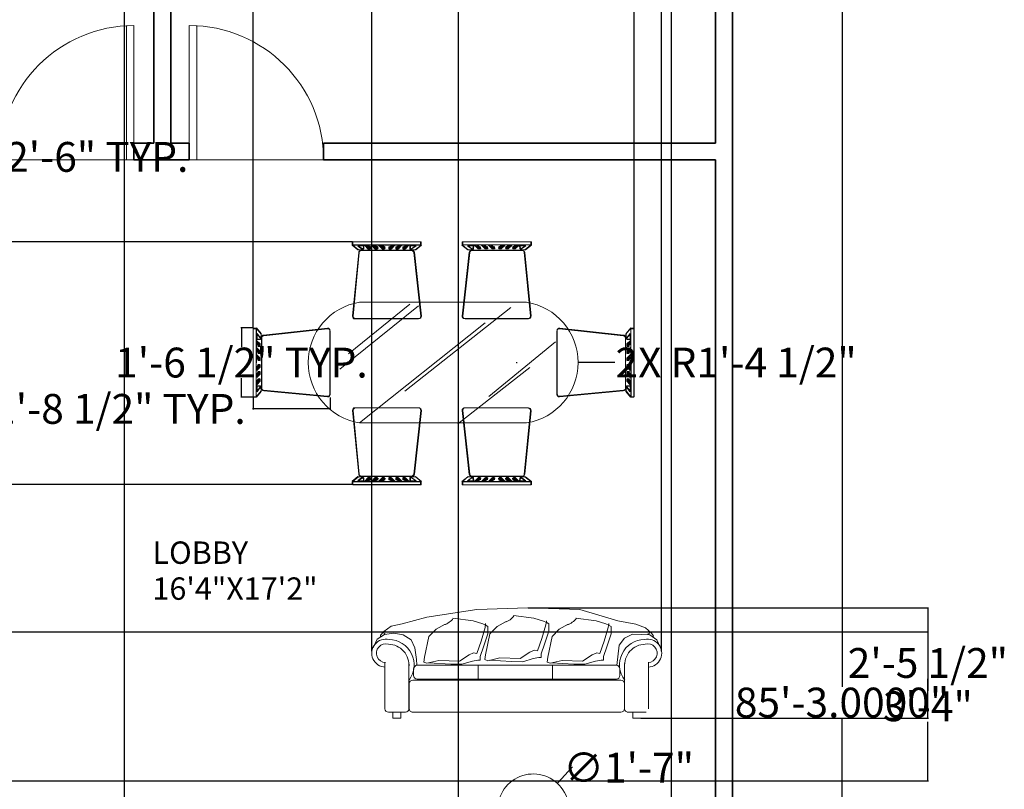
# Model space of a CAD drawing. Units: inches. Extents: x -438 to 102, y -60 to 1091.
# Tile 5 of 20: x -162 to 102, y 492 to 699. Entities that reach past the tile are written whole.
import ezdxf

# ---------------------------------------------------------------- set-up
doc = ezdxf.new("R2010")
doc.units = ezdxf.units.IN
doc.header["$MEASUREMENT"] = 0
for name, color, linetype, lineweight, true_color in [('A-ANNO-DIMS', 217, 'Continuous', 18, 0x93278f), ('A-DOOR', 30, 'Continuous', 18, 0xf26722), ('A-WALL', 2, 'Continuous', 35, 0xf1eb1f), ('C-PROP', 2, 'Continuous', 35, 0xf1eb1f)]:
    doc.layers.add(name, color=color, linetype=linetype, lineweight=lineweight, true_color=true_color)
doc.layers.add('A-AREA-IDEN', color=4, linetype='Continuous', lineweight=18)
doc.layers.add('Furniture', color=7, linetype='Continuous', lineweight=15)
doc.styles.get("Standard").update_dxf_attribs({"font": 'arial.ttf'})
doc.dimstyles.get("Standard").update_dxf_attribs({"dimtxt": 8, "dimasz": 0.18, "dimexe": 0.18, "dimexo": 0.0625, "dimgap": 0.09, "dimtad": 0, "dimtih": 1, "dimtoh": 1, "dimdec": 4, "dimzin": 0, "dimdsep": 46, "dimlunit": 3, "dimtxsty": 'Standard', "dimcen": 0.09, "dimadec": 0, "dimazin": 0, "dimtfac": 1, "dimtdec": 4, "dimtofl": 0, "dimtmove": 0, "dimatfit": 3, "dimfxl": 1, "dimtolj": 1, "dimtzin": 0, "dimarcsym": 0})

# ---------------------------------------------------------------- blocks, each defined once
blk = doc.blocks.new('*D5')
at = {"layer": 'A-ANNO-DIMS', "color": 0, "lineweight": -2, "transparency": 16777216}
for p, q in [((28.92, 1027), (58.42, 1027)), ((58.24, 1026.82), (58.24, 519.68)), ((58.24, 4.18), (58.24, 511.32)), ((28.92, 4), (58.42, 4))]:
    blk.add_line(p, q, dxfattribs=at)
at = {"layer": 'A-ANNO-DIMS', "color": 0, "transparency": 16777216}
for points in [[(58.21, 1026.82), (58.27, 1026.82), (58.24, 1027)], [(58.21, 4.18), (58.27, 4.18), (58.24, 4)]]:
    blk.add_solid(points, dxfattribs=at)
at = {"layer": 'Defpoints', "color": 0, "transparency": 16777216}
for p in [(28.85, 1027), (28.85, 4), (58.24, 4)]:
    blk.add_point(p, dxfattribs=at)
at = {"layer": 'A-ANNO-DIMS', "color": 0, "transparency": 16777216, "insert": (58.24, 515.5), "char_height": 8, "attachment_point": 5}
blk.add_mtext('\\A1;85\'-3.0000"', dxfattribs=at)
blk = doc.blocks.new('DOOR-SWING-36')
for p, q in [((-36, 0), (0, 0)), ((-2, 0), (-2, -36)), ((0, 0), (0, -36))]:
    blk.add_line(p, q)
blk.add_arc((0, 0), 36, 180, 270)
blk = doc.blocks.new('CHAIR-DINING')
for p, q in [((-10.32, -8.58, -3.57), (-10.34, 8.44, -3.57)), ((-10.26, -8.42, -3.57), (-10.28, 8.6, -3.57)), ((-9.64, 9.07, -3.57), (7.45, 7.21, -3.57)), ((-9.58, 9.23, -3.57), (7.51, 7.37, -3.57)), ((9.39, 9.16, -3.57), (8.13, 7.59, -3.57)), ((9.45, 9.32, -3.57), (8.19, 7.75, -3.57)), ((10.27, 9.04, -3.57), (9.45, 9.03, -3.57)), ((9.45, 9.03, -3.57), (9.47, -9.32, -3.57)), ((10.33, 9.2, -3.57), (9.51, 9.2, -3.57)), ((9.51, 9.2, -3.57), (9.53, -9.16, -3.57)), ((10.28, -9.32, -3.57), (10.27, 9.04, -3.57)), ((10.34, -9.16, -3.57), (10.33, 9.2, -3.57)), ((8.01, 6.58, -3.57), (8.02, -6.93, -3.57)), ((8.07, 6.75, -3.57), (8.08, -6.76, -3.57)), ((8.13, 7.59, -3.57), (8.2, 6.27, -3.57)), ((8.19, 7.75, -3.57), (8.25, 6.43, -3.57)), ((8.2, 6.27, -3.57), (9.2, 7.65, -3.57)), ((8.25, 6.43, -3.57), (9.26, 7.81, -3.57)), ((9.26, 6.14, -3.57), (8.38, 6.2, -3.57)), ((9.33, 5.77, -3.57), (8.39, 4.82, -3.57)), ((9.32, 6.3, -3.57), (8.44, 6.37, -3.57)), ((9.39, 5.93, -3.57), (8.44, 4.98, -3.57)), ((8.45, 4.48, -3.57), (9.32, 5.43, -3.57)), ((9.2, 7.65, -3.57), (9.26, 6.14, -3.57)), ((9.26, 7.81, -3.57), (9.32, 6.3, -3.57)), ((9.32, 5.43, -3.57), (9.32, 5.05, -3.57)), ((8.39, 4.32, -3.57), (9.26, 5.26, -3.57)), ((8.39, 4.82, -3.57), (8.39, 4.32, -3.57)), ((9.33, 3.88, -3.57), (8.39, 2.94, -3.57)), ((8.39, 2.43, -3.57), (9.27, 3.38, -3.57)), ((8.39, 2.94, -3.57), (8.39, 2.43, -3.57)), ((8.44, 4.98, -3.57), (8.45, 4.48, -3.57)), ((9.01, 4.32, -3.57), (8.45, 4.26, -3.57)), ((9.39, 4.04, -3.57), (8.45, 3.1, -3.57)), ((8.45, 2.6, -3.57), (9.33, 3.54, -3.57)), ((8.45, 3.1, -3.57), (8.45, 2.6, -3.57)), ((9.07, 4.48, -3.57), (8.51, 4.42, -3.57)), ((9.26, 4.89, -3.57), (8.89, 4.45, -3.57)), ((8.89, 4.45, -3.57), (9.01, 4.32, -3.57)), ((9.27, 3, -3.57), (8.89, 2.56, -3.57)), ((9.32, 5.05, -3.57), (8.95, 4.61, -3.57)), ((8.95, 4.61, -3.57), (9.07, 4.48, -3.57)), ((9.33, 3.16, -3.57), (8.95, 2.72, -3.57)), ((8.95, 2.72, -3.57), (9.08, 2.6, -3.57)), ((9.26, 5.26, -3.57), (9.26, 4.89, -3.57)), ((9.27, 3.38, -3.57), (9.27, 3, -3.57)), ((9.33, 3.54, -3.57), (9.33, 3.16, -3.57)), ((9.33, 1.99, -3.57), (8.39, 1.05, -3.57)), ((8.39, 0.55, -3.57), (9.27, 1.49, -3.57)), ((8.39, 1.05, -3.57), (8.39, 0.55, -3.57)), ((9.02, 2.43, -3.57), (8.45, 2.37, -3.57)), ((9.39, 2.16, -3.57), (8.45, 1.21, -3.57)), ((8.45, 0.71, -3.57), (9.33, 1.65, -3.57)), ((8.45, 1.21, -3.57), (8.45, 0.71, -3.57)), ((9.02, 0.55, -3.57), (8.45, 0.49, -3.57)), ((9.08, 2.6, -3.57), (8.51, 2.53, -3.57)), ((9.08, 0.71, -3.57), (8.51, 0.65, -3.57)), ((8.89, 2.56, -3.57), (9.02, 2.43, -3.57)), ((9.27, 1.11, -3.57), (8.89, 0.67, -3.57)), ((8.89, 0.67, -3.57), (9.02, 0.55, -3.57)), ((9.33, 1.28, -3.57), (8.95, 0.84, -3.57)), ((8.95, 0.84, -3.57), (9.08, 0.71, -3.57)), ((9.27, 1.49, -3.57), (9.27, 1.11, -3.57)), ((9.33, 1.65, -3.57), (9.33, 1.28, -3.57)), ((8.39, -1.21, -3.57), (8.39, -0.71, -3.57)), ((8.39, -0.71, -3.57), (9.27, -1.65, -3.57)), ((9.33, -2.15, -3.57), (8.39, -1.21, -3.57)), ((8.39, -3.1, -3.57), (8.39, -2.59, -3.57)), ((8.39, -2.59, -3.57), (9.27, -3.54, -3.57)), ((8.45, -1.05, -3.57), (8.45, -0.55, -3.57)), ((8.45, -0.55, -3.57), (9.33, -1.49, -3.57)), ((9.02, -0.71, -3.57), (8.45, -0.65, -3.57)), ((9.39, -1.99, -3.57), (8.45, -1.05, -3.57)), ((8.45, -2.94, -3.57), (8.45, -2.43, -3.57)), ((8.45, -2.43, -3.57), (9.33, -3.37, -3.57)), ((9.02, -2.59, -3.57), (8.45, -2.53, -3.57)), ((9.08, -0.55, -3.57), (8.51, -0.48, -3.57)), ((9.08, -2.43, -3.57), (8.51, -2.37, -3.57)), ((8.89, -0.83, -3.57), (9.02, -0.71, -3.57)), ((9.27, -1.27, -3.57), (8.89, -0.83, -3.57)), ((8.89, -2.72, -3.57), (9.02, -2.59, -3.57)), ((8.95, -0.67, -3.57), (9.08, -0.55, -3.57)), ((9.33, -1.11, -3.57), (8.95, -0.67, -3.57)), ((8.95, -2.56, -3.57), (9.08, -2.43, -3.57)), ((9.33, -3, -3.57), (8.95, -2.56, -3.57)), ((9.27, -1.65, -3.57), (9.27, -1.27, -3.57)), ((9.33, -1.49, -3.57), (9.33, -1.11, -3.57)), ((9.34, -4.04, -3.57), (8.39, -3.1, -3.57)), ((8.39, -4.98, -3.57), (8.39, -4.48, -3.57)), ((8.39, -4.48, -3.57), (9.27, -5.42, -3.57)), ((9.34, -5.93, -3.57), (8.39, -4.98, -3.57)), ((9.39, -3.88, -3.57), (8.45, -2.94, -3.57)), ((8.45, -4.82, -3.57), (8.45, -4.32, -3.57)), ((8.45, -4.32, -3.57), (9.33, -5.26, -3.57)), ((9.4, -5.76, -3.57), (8.45, -4.82, -3.57)), ((9.02, -4.48, -3.57), (8.46, -4.42, -3.57)), ((9.08, -4.32, -3.57), (8.52, -4.26, -3.57)), ((9.27, -3.16, -3.57), (8.89, -2.72, -3.57)), ((8.9, -4.61, -3.57), (9.02, -4.48, -3.57)), ((9.27, -5.05, -3.57), (8.9, -4.61, -3.57)), ((8.96, -4.44, -3.57), (9.08, -4.32, -3.57)), ((9.33, -4.88, -3.57), (8.96, -4.44, -3.57)), ((9.27, -3.54, -3.57), (9.27, -3.16, -3.57)), ((9.27, -5.42, -3.57), (9.27, -5.05, -3.57)), ((9.33, -3.37, -3.57), (9.33, -3, -3.57)), ((9.33, -5.26, -3.57), (9.33, -4.88, -3.57)), ((7.45, -7.55, -3.57), (-9.64, -9.21, -3.57)), ((7.51, -7.39, -3.57), (-9.58, -9.04, -3.57)), ((8.14, -7.75, -3.57), (8.21, -6.43, -3.57)), ((9.4, -9.32, -3.57), (8.14, -7.75, -3.57)), ((8.2, -7.59, -3.57), (8.27, -6.27, -3.57)), ((9.46, -9.16, -3.57), (8.2, -7.59, -3.57)), ((8.21, -6.43, -3.57), (9.21, -7.81, -3.57)), ((8.27, -6.27, -3.57), (9.27, -7.65, -3.57)), ((9.27, -6.3, -3.57), (8.39, -6.37, -3.57)), ((9.33, -6.14, -3.57), (8.45, -6.2, -3.57)), ((9.21, -7.81, -3.57), (9.27, -6.3, -3.57)), ((9.27, -7.65, -3.57), (9.33, -6.14, -3.57)), ((9.47, -9.32, -3.57), (10.28, -9.32, -3.57)), ((9.53, -9.16, -3.57), (10.34, -9.16, -3.57))]:
    blk.add_line(p, q)
for centre, start, end in [((-9.71, 8.44, -3.57), 83.7931, 180.0502), ((-9.65, 8.6, -3.57), 83.7931, 180.0502), ((7.38, 6.58, -3.57), 0.0502, 83.7931), ((7.44, 6.75, -3.57), 0.0502, 83.7931), ((7.39, -6.93, -3.57), 275.5303, 0.0502), ((7.45, -6.76, -3.57), 275.5303, 0.0502), ((-9.7, -8.58, -3.57), 180.0502, 275.5303), ((-9.64, -8.42, -3.57), 180.0502, 275.5303)]:
    blk.add_arc(centre, 0.629, start, end)
blk = doc.blocks.new('*D14')
at = {"layer": 'A-ANNO-DIMS', "color": 0, "lineweight": -2, "transparency": 16777216}
for p, q in [((-99.6, 597.28), (-99.6, 594.06)), ((-78.92, 597.28), (-78.92, 594.06)), ((-99.6, 594.24), (-99.78, 594.24)), ((-79.1, 594.24), (-99.42, 594.24))]:
    blk.add_line(p, q, dxfattribs=at)
at = {"layer": 'A-ANNO-DIMS', "color": 0, "transparency": 16777216}
for points in [[(-99.42, 594.27), (-99.42, 594.21), (-99.6, 594.24)], [(-79.1, 594.27), (-79.1, 594.21), (-78.92, 594.24)]]:
    blk.add_solid(points, dxfattribs=at)
at = {"layer": 'Defpoints', "color": 0, "transparency": 16777216}
for p in [(-99.6, 597.34), (-78.92, 597.34), (-99.6, 594.24)]:
    blk.add_point(p, dxfattribs=at)
at = {"layer": 'A-ANNO-DIMS', "color": 0, "transparency": 16777216, "insert": (-152.46, 594.24), "char_height": 8, "attachment_point": 5}
blk.add_mtext('\\A1;CHAIR 1\'-8 1/2" TYP.', dxfattribs=at)
blk = doc.blocks.new('*D15')
at = {"layer": 'A-ANNO-DIMS', "color": 0, "lineweight": -2, "transparency": 16777216}
for p, q in [((-99.66, 615.98), (-102.88, 615.98)), ((-102.7, 615.8), (-102.7, 610.89)), ((-102.7, 597.52), (-102.7, 602.44)), ((-99.66, 597.34), (-102.88, 597.34))]:
    blk.add_line(p, q, dxfattribs=at)
at = {"layer": 'A-ANNO-DIMS', "color": 0, "transparency": 16777216}
for points in [[(-102.73, 615.8), (-102.67, 615.8), (-102.7, 615.98)], [(-102.73, 597.52), (-102.67, 597.52), (-102.7, 597.34)]]:
    blk.add_solid(points, dxfattribs=at)
at = {"layer": 'Defpoints', "color": 0, "transparency": 16777216}
for p in [(-102.7, 615.98), (-99.6, 615.98), (-99.6, 597.34)]:
    blk.add_point(p, dxfattribs=at)
at = {"layer": 'A-ANNO-DIMS', "color": 0, "transparency": 16777216, "insert": (-102.7, 606.66), "char_height": 8, "attachment_point": 5}
blk.add_mtext('\\A1;1\'-6 1/2" TYP.', dxfattribs=at)
blk = doc.blocks.new('*D22')
at = {"layer": 'A-ANNO-DIMS', "color": 0, "lineweight": -2, "transparency": 16777216}
for p, q in [((-230.65, 657.36), (-230.65, 661.98)), ((-230.47, 661.8), (-200.83, 661.8)), ((-200.65, 657.36), (-200.65, 661.98)), ((-200.65, 661.8), (-200.47, 661.8))]:
    blk.add_line(p, q, dxfattribs=at)
at = {"layer": 'A-ANNO-DIMS', "color": 0, "transparency": 16777216}
for points in [[(-230.47, 661.83), (-230.47, 661.77), (-230.65, 661.8)], [(-200.83, 661.83), (-200.83, 661.77), (-200.65, 661.8)]]:
    blk.add_solid(points, dxfattribs=at)
at = {"layer": 'Defpoints', "color": 0, "transparency": 16777216}
for p in [(-200.65, 661.8), (-230.65, 657.3), (-200.65, 657.3)]:
    blk.add_point(p, dxfattribs=at)
at = {"layer": 'A-ANNO-DIMS', "color": 0, "transparency": 16777216, "insert": (-157.88, 661.8), "char_height": 8, "attachment_point": 5}
blk.add_mtext('\\A1;DOOR 2\'-6" TYP.', dxfattribs=at)
blk = doc.blocks.new('*D37')
at = {"layer": 'A-ANNO-DIMS', "color": 0, "lineweight": -2, "transparency": 16777216}
for p, q in [((-179.8, 234.94), (-179.8, 1079.58)), ((-179.62, 1079.4), (-176.98, 1079.4)), ((-134.26, 1079.4), (-136.9, 1079.4)), ((-134.08, 234.94), (-134.08, 1079.58))]:
    blk.add_line(p, q, dxfattribs=at)
at = {"layer": 'A-ANNO-DIMS', "color": 0, "transparency": 16777216}
for points in [[(-179.62, 1079.43), (-179.62, 1079.37), (-179.8, 1079.4)], [(-134.26, 1079.43), (-134.26, 1079.37), (-134.08, 1079.4)]]:
    blk.add_solid(points, dxfattribs=at)
at = {"layer": 'Defpoints', "color": 0, "transparency": 16777216}
for p in [(-134.08, 1079.4), (-179.8, 234.88), (-134.08, 234.88)]:
    blk.add_point(p, dxfattribs=at)
at = {"layer": 'A-ANNO-DIMS', "color": 0, "transparency": 16777216, "insert": (-156.94, 1079.4), "char_height": 8, "attachment_point": 5}
blk.add_mtext('\\A1;3\'-9 1/2"', dxfattribs=at)
blk = doc.blocks.new('*D45')
at = {"layer": 'A-ANNO-DIMS', "color": 0, "lineweight": -2, "transparency": 16777216}
for p, q in [((-99.58, 615.92), (-99.58, 1079.58)), ((-99.4, 1079.4), (-59.27, 1079.4)), ((2.32, 1079.4), (-37.82, 1079.4)), ((2.5, 615.92), (2.5, 1079.58))]:
    blk.add_line(p, q, dxfattribs=at)
at = {"layer": 'A-ANNO-DIMS', "color": 0, "transparency": 16777216}
for points in [[(-99.4, 1079.43), (-99.4, 1079.37), (-99.58, 1079.4)], [(2.32, 1079.43), (2.32, 1079.37), (2.5, 1079.4)]]:
    blk.add_solid(points, dxfattribs=at)
at = {"layer": 'Defpoints', "color": 0, "transparency": 16777216}
for p in [(2.5, 1079.4), (-99.58, 615.86), (2.5, 615.86)]:
    blk.add_point(p, dxfattribs=at)
at = {"layer": 'A-ANNO-DIMS', "color": 0, "transparency": 16777216, "insert": (-48.54, 1079.4), "char_height": 8, "attachment_point": 5}
blk.add_mtext('\\A1;8\'-6"', dxfattribs=at)
blk = doc.blocks.new('*D46')
at = {"layer": 'A-ANNO-DIMS', "color": 0, "lineweight": -2, "transparency": 16777216}
for p, q in [((-72.95, 639.04), (-414.94, 639.04)), ((-414.76, 638.86), (-414.76, 610.65)), ((-414.76, 574.12), (-414.76, 602.33)), ((-73.11, 573.94), (-414.94, 573.94))]:
    blk.add_line(p, q, dxfattribs=at)
at = {"layer": 'A-ANNO-DIMS', "color": 0, "transparency": 16777216}
for points in [[(-414.79, 638.86), (-414.73, 638.86), (-414.76, 639.04)], [(-414.79, 574.12), (-414.73, 574.12), (-414.76, 573.94)]]:
    blk.add_solid(points, dxfattribs=at)
at = {"layer": 'Defpoints', "color": 0, "transparency": 16777216}
for p in [(-414.76, 639.04), (-72.89, 639.04), (-73.05, 573.94)]:
    blk.add_point(p, dxfattribs=at)
at = {"layer": 'A-ANNO-DIMS', "color": 0, "transparency": 16777216, "insert": (-414.76, 606.49), "char_height": 8, "attachment_point": 5}
blk.add_mtext('\\A1;5\'-5"', dxfattribs=at)
blk = doc.blocks.new('*D47')
at = {"layer": 'A-ANNO-DIMS', "color": 0, "lineweight": -2, "transparency": 16777216}
for p, q in [((-67.74, 529.33), (-67.74, 1079.58)), ((-67.56, 1079.4), (-48.98, 1079.4)), ((9.73, 1079.4), (-8.85, 1079.4)), ((9.91, 529.33), (9.91, 1079.58))]:
    blk.add_line(p, q, dxfattribs=at)
at = {"layer": 'A-ANNO-DIMS', "color": 0, "transparency": 16777216}
for points in [[(-67.56, 1079.43), (-67.56, 1079.37), (-67.74, 1079.4)], [(9.73, 1079.43), (9.73, 1079.37), (9.91, 1079.4)]]:
    blk.add_solid(points, dxfattribs=at)
at = {"layer": 'Defpoints', "color": 0, "transparency": 16777216}
for p in [(9.91, 1079.4), (-67.74, 529.27), (9.91, 529.27)]:
    blk.add_point(p, dxfattribs=at)
at = {"layer": 'A-ANNO-DIMS', "color": 0, "transparency": 16777216, "insert": (-28.91, 1079.4), "char_height": 8, "attachment_point": 5}
blk.add_mtext('\\A1;6\'-5 1/2"', dxfattribs=at)
blk = doc.blocks.new('*D48')
at = {"layer": 'A-ANNO-DIMS', "color": 0, "lineweight": -2, "transparency": 16777216}
for p, q in [((-25.85, 540.93), (81.43, 540.93)), ((81.25, 540.75), (81.25, 530.34)), ((81.25, 511.48), (81.25, 521.89)), ((4.34, 511.3), (81.43, 511.3))]:
    blk.add_line(p, q, dxfattribs=at)
at = {"layer": 'A-ANNO-DIMS', "color": 0, "transparency": 16777216}
for points in [[(81.22, 540.75), (81.28, 540.75), (81.25, 540.93)], [(81.22, 511.48), (81.28, 511.48), (81.25, 511.3)]]:
    blk.add_solid(points, dxfattribs=at)
at = {"layer": 'Defpoints', "color": 0, "transparency": 16777216}
for p in [(-25.91, 540.93), (4.28, 511.3), (81.25, 511.3)]:
    blk.add_point(p, dxfattribs=at)
at = {"layer": 'A-ANNO-DIMS', "color": 0, "transparency": 16777216, "insert": (81.25, 526.12), "char_height": 8, "attachment_point": 5}
blk.add_mtext('\\A1;2\'-5 1/2"', dxfattribs=at)
blk = doc.blocks.new('*D49')
at = {"layer": 'A-ANNO-DIMS', "color": 0, "lineweight": -2, "transparency": 16777216}
for p, q in [((-44.57, 339.86), (-44.57, 1079.58)), ((-44.39, 1079.4), (-26.89, 1079.4)), ((12.37, 1079.4), (-5.13, 1079.4)), ((12.55, 312.51), (12.55, 1079.58))]:
    blk.add_line(p, q, dxfattribs=at)
at = {"layer": 'A-ANNO-DIMS', "color": 0, "transparency": 16777216}
for points in [[(-44.39, 1079.43), (-44.39, 1079.37), (-44.57, 1079.4)], [(12.37, 1079.43), (12.37, 1079.37), (12.55, 1079.4)]]:
    blk.add_solid(points, dxfattribs=at)
at = {"layer": 'Defpoints', "color": 0, "transparency": 16777216}
for p in [(12.55, 1079.4), (-44.57, 339.79), (12.55, 312.44)]:
    blk.add_point(p, dxfattribs=at)
at = {"layer": 'A-ANNO-DIMS', "color": 0, "transparency": 16777216, "insert": (-16.01, 1079.4), "char_height": 8, "attachment_point": 5}
blk.add_mtext('\\A1;4\'-9"', dxfattribs=at)
blk = doc.blocks.new('*D60')
at = {"layer": 'A-ANNO-DIMS', "color": 0, "lineweight": -2, "transparency": 16777216}
for p, q in [((-192.58, 534.5), (81.43, 534.5)), ((81.25, 534.32), (81.25, 518.68)), ((81.25, 494.68), (81.25, 510.32)), ((-192.58, 494.5), (81.43, 494.5))]:
    blk.add_line(p, q, dxfattribs=at)
at = {"layer": 'A-ANNO-DIMS', "color": 0, "transparency": 16777216}
for points in [[(81.22, 534.32), (81.28, 534.32), (81.25, 534.5)], [(81.22, 494.68), (81.28, 494.68), (81.25, 494.5)]]:
    blk.add_solid(points, dxfattribs=at)
at = {"layer": 'Defpoints', "color": 0, "transparency": 16777216}
for p in [(-192.65, 534.5), (81.25, 534.5), (-192.65, 494.5)]:
    blk.add_point(p, dxfattribs=at)
at = {"layer": 'A-ANNO-DIMS', "color": 0, "transparency": 16777216, "insert": (81.25, 514.5), "char_height": 8, "attachment_point": 5}
blk.add_mtext('\\A1;3\'-4"', dxfattribs=at)
blk = doc.blocks.new('*D62')
at = {"layer": 'A-ANNO-DIMS', "color": 0, "lineweight": -2, "transparency": 16777216}
for p, q in [((-14.2, 498.06), (-17.94, 493.99)), ((-14.02, 498.06), (-14.2, 498.06)), ((-24.59, 486.85), (-24.41, 486.85)), ((-24.5, 486.76), (-24.5, 486.94))]:
    blk.add_line(p, q, dxfattribs=at)
at = {"layer": 'A-ANNO-DIMS', "color": 0, "transparency": 16777216}
blk.add_solid([(-17.96, 494.01), (-17.92, 493.97), (-18.06, 493.86)], dxfattribs=at)
at = {"layer": 'Defpoints', "color": 0, "transparency": 16777216}
for p in [(-18.06, 493.86), (-30.94, 479.85)]:
    blk.add_point(p, dxfattribs=at)
at = {"layer": 'A-ANNO-DIMS', "color": 0, "transparency": 16777216, "insert": (1.06, 498.06), "char_height": 8, "attachment_point": 5}
blk.add_mtext('\\A1;∅1\'-7"', dxfattribs=at)
blk = doc.blocks.new('*D64')
at = {"layer": 'A-ANNO-DIMS', "color": 0, "lineweight": -2, "transparency": 16777216}
for p, q in [((-28.97, 606.66), (-28.79, 606.66)), ((-28.88, 606.57), (-28.88, 606.75)), ((-2.67, 606.66), (-12.32, 606.66))]:
    blk.add_line(p, q, dxfattribs=at)
at = {"layer": 'A-ANNO-DIMS', "color": 0, "transparency": 16777216}
blk.add_solid([(-12.32, 606.69), (-12.32, 606.63), (-12.5, 606.66)], dxfattribs=at)
at = {"layer": 'Defpoints', "color": 0, "transparency": 16777216}
for p in [(-28.88, 606.66), (-12.5, 606.66)]:
    blk.add_point(p, dxfattribs=at)
at = {"layer": 'A-ANNO-DIMS', "color": 0, "transparency": 16777216, "insert": (29.86, 606.66), "char_height": 8, "attachment_point": 5}
blk.add_mtext('\\A1;2X R1\'-4 1/2"', dxfattribs=at)

msp = doc.modelspace()

# ---------------------------------------------------------------- linework, layer by layer
at = {"layer": 'A-WALL'}
for p, q in [((-126.14649, 665.49939), (-126.14649, 839.49939)), ((-121.64649, 665.49939), (-121.64649, 839.49939)), ((24.35351, 665.49939), (24.35351, 839.49939)), ((-126.14649, 665.49939), (-131.50148, 665.49939)), ((-131.50148, 665.49939), (-131.50148, 660.99939)), ((-116.66828, 665.49939), (-121.64649, 665.49939)), ((-116.66828, 665.49939), (-116.66828, 660.99939)), ((24.35351, 665.49939), (-80.66828, 665.49939)), ((-80.66828, 665.49939), (-80.66828, 660.99939)), ((-116.66828, 660.99939), (-131.50148, 660.99939)), ((24.35351, 660.99939), (-80.66828, 660.99939)), ((24.35351, 454.99939), (24.35351, 660.99939))]:
    msp.add_line(p, q, dxfattribs=at)
at = {"layer": 'C-PROP'}
msp.add_line((28.85351, 3.99939), (28.85351, 1026.99939), dxfattribs=at)
at = {"layer": 'Furniture'}
for p, q in [((-26.28085, 622.83125), (-71.04401, 622.83125)), ((-76.34553, 604.90748), (-55.24223, 621.86128)), ((-74.0517, 609.03138), (-57.53606, 622.31951)), ((-58.91238, 598.95074), (-30.46881, 621.40308)), ((-71.04401, 590.4884), (-37.35031, 617.27918)), ((-36.4328, 597.5761), (-18.54088, 612.23885)), ((-44.69058, 590.24472), (-25.42239, 605.36569)), ((-71.04401, 590.4884), (-26.28085, 590.4884)), ((-24.3199, 538.09972), (-29.76556, 538.81177)), ((-1.83974, 537.45232), (-12.008, 540.47967)), ((-48.11122, 536.56522), (-50.5192, 535.1793)), ((-40.64478, 537.40569), (-46.09044, 538.11774)), ((-38.04282, 536.59165), (-40.64478, 537.40569)), ((-38.49439, 531.95431), (-37.41352, 535.67471)), ((-37.25962, 536.27102), (-38.04282, 536.59165)), ((-37.41352, 535.67471), (-37.26101, 536.69642)), ((-37.26101, 536.69642), (-37.25962, 536.27102)), ((-34.19432, 535.87333), (-36.14173, 533.9403)), ((-31.78634, 537.25925), (-34.19432, 535.87333)), ((-21.71794, 537.28568), (-24.3199, 538.09972)), ((-22.16951, 532.64834), (-21.08863, 536.36873)), ((-20.93474, 536.96505), (-21.71794, 537.28568)), ((-21.08863, 536.36873), (-20.93613, 537.39045)), ((-20.93613, 537.39045), (-20.93474, 536.96505)), ((-15.11413, 536.56522), (-17.5221, 535.1793)), ((-7.64769, 537.40569), (-13.09335, 538.11774)), ((-5.04572, 536.59165), (-7.64769, 537.40569)), ((-5.4973, 531.95431), (-4.41642, 535.67471)), ((-4.26253, 536.27102), (-5.04572, 536.59165)), ((-4.41642, 535.67471), (-4.26391, 536.69642)), ((-4.26391, 536.69642), (-4.26253, 536.27102)), ((3.02912, 536.51966), (-1.83974, 537.45232)), ((5.55027, 535.53949), (3.02912, 536.51966)), ((-52.46661, 533.24627), (-53.63065, 527.63402)), ((-50.5192, 535.1793), (-52.46661, 533.24627)), ((-36.14173, 533.9403), (-37.30577, 528.32805)), ((-19.46952, 533.24627), (-20.63356, 527.63402)), ((-17.5221, 535.1793), (-19.46952, 533.24627)), ((2.06701, 533.86484), (-0.0835, 532.73314)), ((6.76052, 533.66847), (2.06701, 533.86484)), ((7.14586, 534.13883), (5.55027, 535.53949)), ((8.60734, 532.36287), (6.76052, 533.66847)), ((7.70988, 533.44102), (7.14586, 534.13883)), ((7.56719, 533.23631), (7.70988, 533.44102)), ((-39.64735, 528.67452), (-38.49439, 531.95431)), ((-23.32247, 529.36855), (-22.16951, 532.64834)), ((-6.65026, 528.67452), (-5.4973, 531.95431)), ((-1.47311, 530.89885), (-2.07965, 525.48157)), ((-0.0835, 532.73314), (-1.47311, 530.89885)), ((9.5637, 530.18661), (8.60734, 532.36287)), ((-44.29816, 526.62205), (-41.71015, 528.34168)), ((-41.71015, 528.34168), (-40.50202, 528.87348)), ((-40.50202, 528.87348), (-39.64735, 528.67452)), ((-37.30577, 528.32805), (-37.46342, 527.02219)), ((-27.97328, 527.31608), (-25.38527, 529.03571)), ((-25.38527, 529.03571), (-24.17714, 529.5675)), ((-24.17714, 529.5675), (-23.32247, 529.36855)), ((-11.30107, 526.62205), (-8.71306, 528.34168)), ((-8.71306, 528.34168), (-7.50493, 528.87348)), ((-7.50493, 528.87348), (-6.65026, 528.67452)), ((-64.24063, 526.25603), (-64.24063, 513.84815)), ((-57.81217, 525.99166), (-57.81217, 513.84815)), ((-55.66896, 525.49137), (-2.21506, 525.49137)), ((-53.63065, 527.63402), (-53.7883, 526.32817)), ((-53.7883, 526.32817), (-52.98731, 526.03419)), ((-52.98731, 526.03419), (-49.76239, 526.76244)), ((-49.76239, 526.76244), (-44.29816, 526.62205)), ((-39.23884, 525.49137), (-39.23884, 521.81712)), ((-37.46342, 527.02219), (-36.66243, 526.72821)), ((-36.66243, 526.72821), (-33.43751, 527.45647)), ((-33.43751, 527.45647), (-27.97328, 527.31608)), ((-20.63356, 527.63402), (-20.79121, 526.32817)), ((-20.79121, 526.32817), (-19.99022, 526.03419)), ((-19.99022, 526.03419), (-16.76529, 526.76244)), ((-19.3499, 525.49137), (-19.3499, 521.81712)), ((-16.76529, 526.76244), (-11.30107, 526.62205)), ((-0.03856, 525.49137), (-0.01615, 525.49137)), ((-0.01615, 525.99166), (-0.01615, 513.84815)), ((6.41231, 526.25603), (6.41231, 513.84815)), ((-56.55373, 524.5509), (-56.55373, 522.75758)), ((-1.27459, 524.5509), (-1.27459, 522.75758)), ((-57.74785, 520.57561), (-57.74785, 513.89229)), ((-56.80738, 521.51608), (-1.02094, 521.51608)), ((-2.21506, 521.81712), (-55.61326, 521.81712)), ((-55.61326, 521.81712), (-2.21506, 521.81712)), ((-0.08047, 520.57561), (-0.08047, 513.89229)), ((-58.75263, 512.90768), (-63.30017, 512.90768)), ((-62.10714, 512.90768), (-62.10714, 511.30191)), ((-59.99319, 511.30191), (-59.99319, 512.90768)), ((-57.02476, 512.95183), (-1.02094, 512.95183)), ((0.63957, 512.95183), (5.7566, 512.95183)), ((0.92431, 512.90768), (5.47185, 512.90768)), ((2.16487, 511.30191), (2.16487, 512.90768)), ((-62.10714, 511.30191), (-59.99319, 511.30191)), ((4.27882, 511.30191), (2.16487, 511.30191))]:
    msp.add_line(p, q, dxfattribs=at)
at = {"layer": 'Furniture', "extrusion": (0, 0, -1)}
for p, q in [((-39.62991, 540.49521), (-25.91384, 540.93064)), ((-25.91384, 540.93064), (-12.008, 540.47967)), ((-59.5896, 536.5953), (-53.0217, 538.4292)), ((-53.0217, 538.4292), (-39.62991, 540.49521)), ((-64.51314, 534.59901), (-62.58848, 536.00978)), ((-62.58848, 536.00978), (-59.5896, 536.5953)), ((-37.38553, 536.33234), (-36.63782, 535.92852)), ((-36.63782, 535.92852), (-36.6601, 533.97478)), ((-21.06065, 537.02637), (-20.31293, 536.62255)), ((-20.31293, 536.62255), (-20.33522, 534.66881)), ((-4.38844, 536.33234), (-3.64072, 535.92852)), ((-3.64072, 535.92852), (-3.66301, 533.97478)), ((-66.36376, 532.46216), (-64.34068, 533.75181)), ((-65.43129, 533.60584), (-64.51314, 534.59901)), ((-65.39551, 533.23631), (-65.43129, 533.60584)), ((-64.34068, 533.75181), (-61.85369, 534.14496)), ((-61.85369, 534.14496), (-59.40449, 533.69607)), ((-59.40449, 533.69607), (-57.24807, 532.28249)), ((-36.6601, 533.97478), (-37.81253, 530.43007)), ((-20.33522, 534.66881), (-21.48765, 531.1241)), ((-3.66301, 533.97478), (-4.81544, 530.43007)), ((-67.39202, 530.18661), (-66.36376, 532.46216)), ((-57.24807, 532.28249), (-56.22151, 530.22411)), ((-37.81253, 530.43007), (-38.71065, 527.85263)), ((-21.48765, 531.1241), (-22.38577, 528.54666)), ((-4.81544, 530.43007), (-5.71356, 527.85263)), ((-56.22151, 530.22411), (-55.75228, 527.09183)), ((-38.71065, 527.85263), (-38.71007, 526.85938)), ((-22.38577, 528.54666), (-22.38519, 527.55341)), ((-5.71356, 527.85263), (-5.71298, 526.85938)), ((-55.69791, 525.64786), (-56.35249, 525.26017)), ((-55.75228, 527.09183), (-55.69791, 525.64786)), ((-46.62906, 525.78999), (-52.5414, 526.16332)), ((-43.66279, 525.76182), (-46.62906, 525.78999)), ((-40.80598, 526.61825), (-43.66279, 525.76182)), ((-39.33414, 526.88305), (-40.80598, 526.61825)), ((-38.71007, 526.85938), (-39.33414, 526.88305)), ((-30.30418, 526.48401), (-36.21652, 526.85735)), ((-27.33791, 526.45585), (-30.30418, 526.48401)), ((-24.4811, 527.31228), (-27.33791, 526.45585)), ((-23.00926, 527.57708), (-24.4811, 527.31228)), ((-22.38519, 527.55341), (-23.00926, 527.57708)), ((-13.63196, 525.78999), (-19.54431, 526.16332)), ((-10.6657, 525.76182), (-13.63196, 525.78999)), ((-7.80889, 526.61825), (-10.6657, 525.76182)), ((-6.33705, 526.88305), (-7.80889, 526.61825)), ((-5.71298, 526.85938), (-6.33705, 526.88305))]:
    msp.add_line(p, q, dxfattribs=at)
at = {"layer": 'Furniture'}
for centre, radius, start, end in [((-68.44448, 606.65983), 16.37903, 99.132079, 260.867921), ((-28.88038, 606.65983), 16.37903, 279.132079, 80.867921), ((-33.5626, 541.69268), 4.89098, 287.4338656, 323.9121988), ((-49.88748, 540.99865), 4.89098, 287.4338656, 323.9121988), ((-16.89038, 540.99865), 4.89098, 287.4338656, 323.9121988), ((-64.04493, 534.29198), 0.47285, 97.1337662, 277.1337662), ((6.21661, 534.29198), 0.47285, 262.8662338, 82.8662338), ((-64.01643, 528.75081), 3.75879, 76.233296, 268.0261658), ((-64.01643, 528.75081), 2.50483, 74.108222, 268.0261658), ((-63.46333, 525.48789), 5.67358, 354.9058451, 88.659022), ((-63.229, 525.60016), 6.8023, 323.2150443, 89.0983641), ((5.37846, 525.63521), 6.76694, 90.7182064, 217.381654), ((5.63501, 525.48789), 5.67358, 91.340978, 185.0941549), ((6.18811, 528.75081), 3.75879, 271.9738342, 103.766704), ((6.18811, 528.75081), 2.50483, 271.9738342, 105.891778), ((-55.61326, 524.5509), 0.94047, 90, 180), ((-2.21506, 524.5509), 0.94047, 0, 90), ((-55.61326, 522.75758), 0.94047, 180, 270), ((-2.21506, 522.75758), 0.94047, 270, 0), ((-56.80738, 520.57561), 0.94047, 90, 180), ((-1.02094, 520.57561), 0.94047, 0, 90), ((-63.30017, 513.84815), 0.94047, 180, 270), ((-58.75263, 513.84815), 0.94047, 270, 0), ((-56.80738, 513.89229), 0.94047, 180, 270), ((-1.02094, 513.89229), 0.94047, 270, 0), ((0.92431, 513.84815), 0.94047, 180, 270), ((-24.50081, 486.85219), 9.51534, 259.3798673, 195.4129607)]:
    msp.add_arc(centre, radius, start, end, dxfattribs=at)

# ---------------------------------------------------------------- block references
at = {"layer": 'A-DOOR', "extrusion": (0, 0, -1), "zscale": -1, "rotation": 180}
msp.add_blockref('DOOR-SWING-36', (131.50148, 660.99939), dxfattribs=at)
at = {"layer": 'A-DOOR', "rotation": 180}
msp.add_blockref('DOOR-SWING-36', (-116.66828, 660.99939), dxfattribs=at)
at = {"layer": 'Furniture', "extrusion": (0, 0, -1), "zscale": -1}
for p, rotation in [((63.72377, 628.70698), 89.94977784564654), ((34.31136, 584.20173), 269.9999999999989)]:
    msp.add_blockref('CHAIR-DINING', p, dxfattribs=dict(at, rotation=rotation))
at = {"layer": 'Furniture'}
for p, rotation in [((-34.31136, 628.71987), 89.99999999999692), ((-63.72377, 584.21462), 269.9497778456449)]:
    msp.add_blockref('CHAIR-DINING', p, dxfattribs=dict(at, rotation=rotation))
at = {"layer": 'Furniture', "extrusion": (0, 0, -1), "zscale": -1}
msp.add_blockref('CHAIR-DINING', (89.25822, 606.66), dxfattribs=at)
at = {"layer": 'Furniture'}
msp.add_blockref('CHAIR-DINING', (-7.83, 606.66), dxfattribs=at)

# ---------------------------------------------------------------- texts
at = {"layer": 'A-AREA-IDEN'}
for s, p in [('LOBBY', (-126.54744, 552.69638)), ('16\'4"X17\'2"', (-126.54744, 543.05791))]:
    msp.add_text(s, height=6, dxfattribs=at).set_placement(p)

# ---------------------------------------------------------------- dimensions: what is measured, and where the dimension line sits
at = {"layer": 'A-ANNO-DIMS'}
for base, p1, p2, picture, middle in [((-134.07948, 1079.39939), (-179.79585, 234.87846), (-134.07948, 234.87846), '*D37', (-156.93767, 1079.39939)), ((9.9115, 1079.39939), (-67.73982, 529.2655), (9.9115, 529.2655), '*D47', (-28.91416, 1079.39939)), ((2.49567, 1079.39939), (-99.58389, 615.85716), (2.49567, 615.85716), '*D45', (-48.54411, 1079.39939)), ((12.55306, 1079.39939), (-44.57214, 339.79496), (12.55306, 312.44261), '*D49', (-16.00954, 1079.39939))]:
    dim = msp.add_linear_dim(base=base, p1=p1, p2=p2, dimstyle='Standard', override={"dimdec": 1, "dimlfac": 1, "dimrnd": 0, "dimzin": 1, "dimdsep": 46, "dimlunit": 4, "dimfrac": 2}, dxfattribs=at)
    dim.commit()
    dim.dimension.update_dxf_attribs({"geometry": picture, "text_midpoint": middle})
for base, p1, p2, override, picture, middle in [((58.24207, 3.99939), (28.85351, 1026.99939), (28.85351, 3.99939), {"dimclrd": 0, "dimclre": 0, "dimclrt": 0}, '*D5', (58.24207, 515.49939)), ((-414.76009, 639.04071), (-73.0511, 573.94064), (-72.889, 639.04071), {"dimdec": 1, "dimlfac": 1, "dimrnd": 0, "dimzin": 1, "dimdsep": 46, "dimlunit": 4, "dimfrac": 2}, '*D46', (-414.76009, 606.49067)), ((81.25351, 511.30191), (-25.91384, 540.93064), (4.27882, 511.30191), {"dimdec": 1, "dimlfac": 1, "dimrnd": 0, "dimzin": 1, "dimdsep": 46, "dimlunit": 4, "dimfrac": 2}, '*D48', (81.25351, 526.11628)), ((81.25351, 534.49939), (-192.64649, 494.49939), (-192.64649, 534.49939), {"dimdec": 1, "dimlfac": 1, "dimrnd": 0, "dimzin": 1, "dimdsep": 46, "dimlunit": 4, "dimfrac": 2}, '*D60', (81.25351, 514.49939))]:
    dim = msp.add_linear_dim(base=base, p1=p1, p2=p2, angle=90, dimstyle='Standard', override=override, dxfattribs=at)
    dim.commit()
    dim.dimension.update_dxf_attribs({"geometry": picture, "text_midpoint": middle})
dim = msp.add_linear_dim(base=(-200.64649, 661.80022), p1=(-230.64649, 657.30022), p2=(-200.64649, 657.30022), text='DOOR <> TYP.', dimstyle='Standard', override={"dimdec": 1, "dimlfac": 1, "dimrnd": 0, "dimzin": 1, "dimdsep": 46, "dimlunit": 4, "dimfrac": 2}, dxfattribs=at)
dim.commit()
dim.dimension.update_dxf_attribs({"geometry": '*D22', "text_midpoint": (-157.87717, 661.80022)})
for base, p1, p2, angle, text, picture, middle in [((-102.70213, 615.98209), (-99.59998, 597.34091), (-99.59998, 615.98209), 90, '<> TYP.', '*D15', (-102.70213, 606.6615)), ((-99.59998, 594.23876), (-78.919, 597.34091), (-99.59998, 597.34091), 180, 'CHAIR <> TYP.', '*D14', (-152.4648, 594.23876))]:
    dim = msp.add_linear_dim(base=base, p1=p1, p2=p2, angle=angle, text=text, dimstyle='Standard', override={"dimdec": 1, "dimlfac": 1, "dimrnd": 0, "dimzin": 1, "dimdsep": 46, "dimlunit": 4, "dimfrac": 2}, dxfattribs=at)
    dim.commit()
    dim.dimension.update_dxf_attribs({"geometry": picture, "text_midpoint": middle})
dim = msp.add_radius_dim(center=(-28.88038, 606.65983), mpoint=(-12.50135, 606.66), text='2X <>', dimstyle='Standard', override={"dimdec": 1, "dimlfac": 1, "dimrnd": 0, "dimzin": 1, "dimdsep": 46, "dimlunit": 4, "dimfrac": 2}, dxfattribs=at)
dim.commit()
dim.dimension.update_dxf_attribs({"geometry": '*D64', "text_midpoint": (-2.67393, 606.6601), "dimtype": 164})
dim = msp.add_diameter_dim_2p(p1=(-30.94177, 479.84822), p2=(-18.05985, 493.85616), dimstyle='Standard', override={"dimdec": 1, "dimlfac": 1, "dimrnd": 0, "dimzin": 1, "dimdsep": 46, "dimlunit": 4, "dimfrac": 2}, dxfattribs=at)
dim.commit()
dim.dimension.update_dxf_attribs({"geometry": '*D62', "text_midpoint": (1.05972, 498.05855), "dimtype": 163})

doc.saveas('drawing.dxf')
